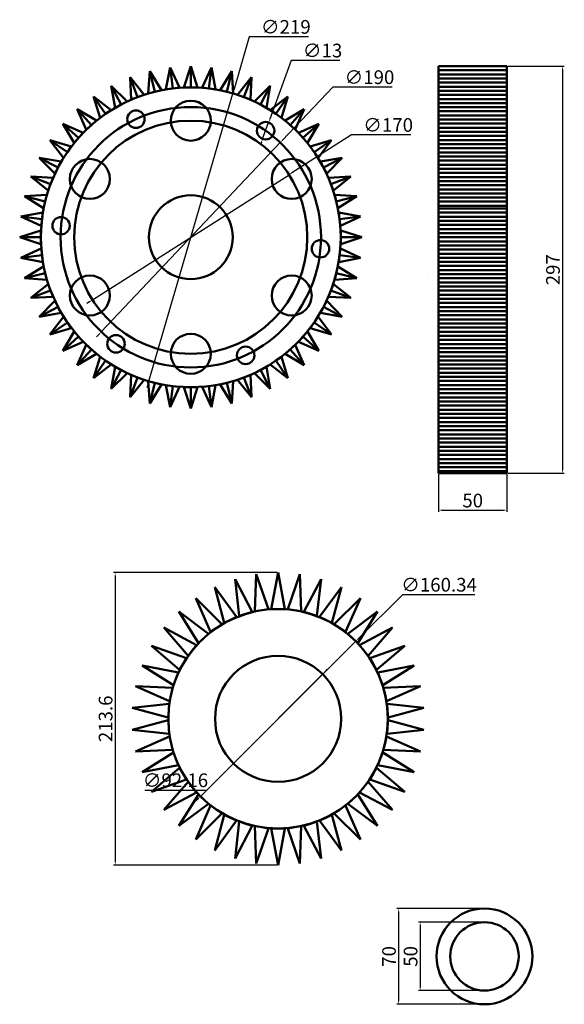
# Model space of a CAD drawing. Units: millimetres. Extents: x 828 to 2987, y 979 to 1807.
# Tile 5 of 6: x 1664 to 2062, y 1028 to 1747. Entities that reach past the tile are written whole.
import ezdxf

# ---------------------------------------------------------------- set-up
doc = ezdxf.new("R2010")
doc.units = ezdxf.units.MM
doc.layers.add('M-DIMS', color=2, linetype='Continuous', lineweight=25)
doc.layers.add('M-OUTL', color=7, linetype='Continuous', lineweight=50)
doc.styles.get("Standard").update_dxf_attribs({"font": 'arial.ttf'})
doc.dimstyles.new('ISO-25', dxfattribs={"dimtxt": 10, "dimasz": 2.5, "dimexe": 1.25, "dimexo": 0.625, "dimtad": 1, "dimtoh": 1, "dimdec": 0, "dimtxsty": 'Standard', "dimcen": 2.5, "dimadec": 0, "dimazin": 0, "dimtfac": 1, "dimtdec": 0, "dimtmove": 0, "dimatfit": 3, "dimfxl": 1, "dimarcsym": 0})

# ---------------------------------------------------------------- blocks, each defined once
blk = doc.blocks.new('*U45')
for p, q in [((-5, -7.75), (0, 7.75)), ((0, -7.75), (0, 7.75)), ((5, -7.75), (0, 7.75)), ((0, -7.75), (-5, -7.75)), ((0, -7.75), (5, -7.75))]:
    blk.add_line(p, q)
blk = doc.blocks.new('*U46')
at = {"layer": 'M-OUTL', "color": 0, "linetype": 'ByBlock', "lineweight": -2, "transparency": 16777216}
for p, rotation in [((1775.03, 1704.64), 6.923076923076879), ((1803.3, 1704.64), 353.0769230769231), ((1747.59, 1697.88), 20.76923076923077), ((1761.1, 1702.09), 13.84615384615382), ((1817.23, 1702.09), 346.1538461538462), ((1830.74, 1697.88), 339.2307692307692), ((1734.67, 1692.07), 27.69230769230768), ((1843.66, 1692.07), 332.3076923076923), ((1722.56, 1684.74), 34.61538461538462), ((1855.77, 1684.74), 325.3846153846154), ((1711.41, 1676.01), 41.53846153846155), ((1866.92, 1676.01), 318.4615384615384), ((1701.4, 1666), 48.46153846153847), ((1876.93, 1666), 311.5384615384616), ((1692.67, 1654.85), 55.38461538461539), ((1885.66, 1654.85), 304.6153846153846), ((1685.34, 1642.74), 62.30769230769233), ((1892.99, 1642.74), 297.6923076923078), ((1679.53, 1629.82), 69.23076923076925), ((1898.8, 1629.82), 290.7692307692308), ((1675.32, 1616.31), 76.15384615384616), ((1903.01, 1616.31), 283.8461538461539), ((1672.77, 1602.38), 83.07692307692308), ((1905.56, 1602.38), 276.923076923077), ((1671.91, 1588.25), 90), ((1906.42, 1588.25), 270.0000000000001), ((1672.77, 1574.11), 96.92307692307695), ((1905.56, 1574.11), 263.0769230769231), ((1675.32, 1560.19), 103.8461538461538), ((1903.01, 1560.19), 256.1538461538462), ((1679.53, 1546.67), 110.7692307692307), ((1898.8, 1546.67), 249.2307692307693), ((1685.34, 1533.76), 117.6923076923077), ((1892.99, 1533.76), 242.3076923076923), ((1692.67, 1521.64), 124.6153846153846), ((1885.66, 1521.64), 235.3846153846154), ((1701.4, 1510.49), 131.5384615384615), ((1876.93, 1510.49), 228.4615384615384), ((1711.41, 1500.48), 138.4615384615385), ((1866.92, 1500.48), 221.5384615384615), ((1722.56, 1491.75), 145.3846153846154), ((1855.77, 1491.75), 214.6153846153847), ((1734.67, 1484.42), 152.3076923076923), ((1843.66, 1484.42), 207.6923076923077), ((1747.59, 1478.61), 159.2307692307692), ((1761.1, 1474.4), 166.1538461538462), ((1817.23, 1474.4), 193.8461538461538), ((1830.74, 1478.61), 200.7692307692307), ((1775.03, 1471.85), 173.0769230769231), ((1789.16, 1470.99), 180), ((1803.3, 1471.85), 186.9230769230768)]:
    blk.add_blockref('*U45', p, dxfattribs=dict(at, rotation=rotation))
blk.add_blockref('*U45', (1789.16, 1705.5), dxfattribs=at)
blk = doc.blocks.new('*U47')
blk.add_circle((0, 0), 14.61)
blk = doc.blocks.new('*U48')
at = {"layer": 'M-OUTL', "color": 0, "linetype": 'ByBlock', "lineweight": -2, "transparency": 16777216}
blk.add_blockref('*U47', (1789.16, 1673.38), dxfattribs=at)
for p, rotation in [((1715.43, 1630.81), 59.99999999999999), ((1862.9, 1630.81), 300), ((1715.43, 1545.68), 120), ((1862.9, 1545.68), 240), ((1789.16, 1503.11), 180)]:
    blk.add_blockref('*U47', p, dxfattribs=dict(at, rotation=rotation))
blk = doc.blocks.new('*U49')
blk.add_circle((0, 0), 6.37)
blk = doc.blocks.new('*U50')
at = {"layer": 'M-OUTL', "color": 0, "linetype": 'ByBlock', "lineweight": -2, "transparency": 16777216}
blk.add_blockref('*U49', (1749.08, 1674.51), dxfattribs=at)
for p, rotation in [((1843.83, 1666.09), 300), ((1694.41, 1596.66), 60), ((1883.92, 1579.83), 239.9999999999999), ((1734.5, 1510.4), 120), ((1829.25, 1501.98), 180)]:
    blk.add_blockref('*U49', p, dxfattribs=dict(at, rotation=rotation))
blk = doc.blocks.new('*D51')
at = {"layer": 'Defpoints', "color": 0, "transparency": 16777216}
for p in [(1970.13, 1415.79), (2020.13, 1415.79), (2020.13, 1388.87)]:
    blk.add_point(p, dxfattribs=at)
at = {"layer": 'M-DIMS', "color": 0, "lineweight": -2, "transparency": 16777216}
for p, q in [((1970.13, 1415.16), (1970.13, 1387.62)), ((2020.13, 1415.16), (2020.13, 1387.62)), ((1972.63, 1388.87), (2017.63, 1388.87))]:
    blk.add_line(p, q, dxfattribs=at)
at = {"layer": 'M-DIMS', "color": 0, "transparency": 16777216}
for points in [[(1972.63, 1389.29), (1972.63, 1388.45), (1970.13, 1388.87)], [(2017.63, 1389.29), (2017.63, 1388.45), (2020.13, 1388.87)]]:
    blk.add_solid(points, dxfattribs=at)
at = {"layer": 'M-DIMS', "color": 0, "transparency": 16777216, "insert": (1995.13, 1394.6), "char_height": 10, "attachment_point": 5}
blk.add_mtext('50', dxfattribs=at)
blk = doc.blocks.new('*D52')
at = {"layer": 'Defpoints', "color": 0, "transparency": 16777216}
for p in [(2020.13, 1713.25), (2020.13, 1415.79), (2060.79, 1415.79)]:
    blk.add_point(p, dxfattribs=at)
at = {"layer": 'M-DIMS', "color": 0, "lineweight": -2, "transparency": 16777216}
for p, q in [((2020.76, 1713.25), (2062.04, 1713.25)), ((2060.79, 1710.75), (2060.79, 1418.29)), ((2020.76, 1415.79), (2062.04, 1415.79))]:
    blk.add_line(p, q, dxfattribs=at)
at = {"layer": 'M-DIMS', "color": 0, "transparency": 16777216}
for points in [[(2060.38, 1710.75), (2061.21, 1710.75), (2060.79, 1713.25)], [(2060.38, 1418.29), (2061.21, 1418.29), (2060.79, 1415.79)]]:
    blk.add_solid(points, dxfattribs=at)
at = {"layer": 'M-DIMS', "color": 0, "transparency": 16777216, "insert": (2055.06, 1564.52), "char_height": 10, "attachment_point": 5, "rotation": 90}
blk.add_mtext('297', dxfattribs=at)
blk = doc.blocks.new('*D53')
at = {"layer": 'Defpoints', "color": 0, "transparency": 16777216}
for p in [(1819.8, 1693.38), (1758.53, 1483.11)]:
    blk.add_point(p, dxfattribs=at)
at = {"layer": 'M-DIMS', "color": 0, "lineweight": -2, "transparency": 16777216}
for p, q in [((1831.82, 1734.62), (1820.5, 1695.78)), ((1875.09, 1734.62), (1831.82, 1734.62)), ((1758.53, 1483.11), (1819.8, 1693.38)), ((1757.83, 1480.71), (1757.13, 1478.31))]:
    blk.add_line(p, q, dxfattribs=at)
at = {"layer": 'M-DIMS', "color": 0, "transparency": 16777216}
for points in [[(1820.1, 1695.9), (1820.9, 1695.66), (1819.8, 1693.38)], [(1757.43, 1480.83), (1758.23, 1480.59), (1758.53, 1483.11)]]:
    blk.add_solid(points, dxfattribs=at)
at = {"layer": 'M-DIMS', "color": 0, "transparency": 16777216, "insert": (1858.59, 1740.63), "char_height": 10, "attachment_point": 5}
blk.add_mtext('∅219', dxfattribs=at)
blk = doc.blocks.new('*D54')
at = {"layer": 'Defpoints', "color": 0, "transparency": 16777216}
for p in [(1854.53, 1657.36), (1723.8, 1519.13)]:
    blk.add_point(p, dxfattribs=at)
at = {"layer": 'M-DIMS', "color": 0, "lineweight": -2, "transparency": 16777216}
for p, q in [((1892.84, 1697.87), (1856.24, 1659.18)), ((1936.17, 1697.87), (1892.84, 1697.87)), ((1723.8, 1519.13), (1854.53, 1657.36)), ((1722.09, 1517.31), (1720.37, 1515.5))]:
    blk.add_line(p, q, dxfattribs=at)
at = {"layer": 'M-DIMS', "color": 0, "transparency": 16777216}
for points in [[(1855.94, 1659.46), (1856.55, 1658.89), (1854.53, 1657.36)], [(1721.78, 1517.6), (1722.39, 1517.03), (1723.8, 1519.13)]]:
    blk.add_solid(points, dxfattribs=at)
at = {"layer": 'M-DIMS', "color": 0, "transparency": 16777216, "insert": (1919.7, 1703.88), "char_height": 10, "attachment_point": 5}
blk.add_mtext('∅190', dxfattribs=at)
blk = doc.blocks.new('*D55')
at = {"layer": 'Defpoints', "color": 0, "transparency": 16777216}
for p in [(1846.01, 1672.08), (1841.65, 1660.1)]:
    blk.add_point(p, dxfattribs=at)
at = {"layer": 'M-DIMS', "color": 0, "lineweight": -2, "transparency": 16777216}
for p, q in [((1862.47, 1717.36), (1846.86, 1674.43)), ((1898.05, 1717.36), (1862.47, 1717.36)), ((1841.65, 1660.1), (1846.01, 1672.08)), ((1840.8, 1657.76), (1839.95, 1655.41))]:
    blk.add_line(p, q, dxfattribs=at)
at = {"layer": 'M-DIMS', "color": 0, "transparency": 16777216}
for points in [[(1846.47, 1674.58), (1847.26, 1674.29), (1846.01, 1672.08)], [(1840.41, 1657.9), (1841.19, 1657.61), (1841.65, 1660.1)]]:
    blk.add_solid(points, dxfattribs=at)
at = {"layer": 'M-DIMS', "color": 0, "transparency": 16777216, "insert": (1885.44, 1723.37), "char_height": 10, "attachment_point": 5}
blk.add_mtext('∅13', dxfattribs=at)
blk = doc.blocks.new('*D56')
at = {"layer": 'Defpoints', "color": 0, "transparency": 16777216}
for p in [(1860.98, 1633.97), (1717.35, 1542.52)]:
    blk.add_point(p, dxfattribs=at)
at = {"layer": 'M-DIMS', "color": 0, "lineweight": -2, "transparency": 16777216}
for p, q in [((1906.52, 1662.97), (1863.09, 1635.32)), ((1949.82, 1662.97), (1906.52, 1662.97)), ((1717.35, 1542.52), (1860.98, 1633.97)), ((1715.24, 1541.18), (1713.13, 1539.83))]:
    blk.add_line(p, q, dxfattribs=at)
at = {"layer": 'M-DIMS', "color": 0, "transparency": 16777216}
for points in [[(1862.86, 1635.67), (1863.31, 1634.96), (1860.98, 1633.97)], [(1715.02, 1541.53), (1715.47, 1540.82), (1717.35, 1542.52)]]:
    blk.add_solid(points, dxfattribs=at)
at = {"layer": 'M-DIMS', "color": 0, "transparency": 16777216, "insert": (1933.35, 1668.98), "char_height": 10, "attachment_point": 5}
blk.add_mtext('∅170', dxfattribs=at)
blk = doc.blocks.new('*U57')
for p, q in [((-5, -13.32), (0, 13.32)), ((5, -13.32), (0, 13.32)), ((0, -13.32), (-5, -13.32)), ((0, -13.32), (5, -13.32))]:
    blk.add_line(p, q)
blk = doc.blocks.new('*U58')
at = {"layer": 'M-OUTL', "color": 0, "linetype": 'ByBlock', "lineweight": -2, "transparency": 16777216}
for p, rotation in [((1825.4, 1325.77), 17.14285714285713), ((1839.02, 1328.88), 8.571428571428495), ((1866.89, 1328.88), 351.4285714285715), ((1880.51, 1325.77), 342.8571428571429), ((1812.39, 1320.67), 25.71428571428572), ((1893.52, 1320.67), 334.2857142857143), ((1800.29, 1313.68), 34.28571428571429), ((1905.62, 1313.68), 325.7142857142857), ((1789.37, 1304.97), 42.85714285714287), ((1916.54, 1304.97), 317.1428571428572), ((1779.86, 1294.72), 51.42857142857143), ((1926.05, 1294.72), 308.5714285714286), ((1771.99, 1283.18), 60), ((1933.92, 1283.18), 300), ((1765.93, 1270.59), 68.57142857142858), ((1939.98, 1270.59), 291.4285714285714), ((1761.81, 1257.24), 77.14285714285714), ((1944.1, 1257.24), 282.8571428571428), ((1759.73, 1243.42), 85.71428571428572), ((1946.18, 1243.42), 274.2857142857143), ((1759.73, 1229.45), 94.28571428571432), ((1946.18, 1229.45), 265.7142857142857), ((1761.81, 1215.63), 102.8571428571428), ((1944.1, 1215.63), 257.1428571428572), ((1765.93, 1202.28), 111.4285714285714), ((1939.98, 1202.28), 248.5714285714286), ((1771.99, 1189.69), 120), ((1933.92, 1189.69), 240), ((1779.86, 1178.15), 128.5714285714286), ((1926.05, 1178.15), 231.4285714285714), ((1789.37, 1167.9), 137.1428571428571), ((1916.54, 1167.9), 222.8571428571428), ((1800.29, 1159.19), 145.7142857142857), ((1905.62, 1159.19), 214.2857142857143), ((1812.39, 1152.21), 154.2857142857143), ((1893.52, 1152.21), 205.7142857142857), ((1825.4, 1147.1), 162.8571428571429), ((1880.51, 1147.1), 197.1428571428571), ((1839.02, 1143.99), 171.4285714285715), ((1852.96, 1142.95), 180), ((1866.89, 1143.99), 188.5714285714286)]:
    blk.add_blockref('*U57', p, dxfattribs=dict(at, rotation=rotation))
blk.add_blockref('*U57', (1852.96, 1329.92), dxfattribs=at)
blk = doc.blocks.new('*D59')
at = {"layer": 'Defpoints', "color": 0, "transparency": 16777216}
for p in [(2003.72, 1097.86), (1941, 1027.86), (2003.72, 1027.86)]:
    blk.add_point(p, dxfattribs=at)
at = {"layer": 'M-DIMS', "color": 0, "lineweight": -2, "transparency": 16777216}
for p, q in [((2003.09, 1097.86), (1939.75, 1097.86)), ((1941, 1095.36), (1941, 1030.36)), ((2003.09, 1027.86), (1939.75, 1027.86))]:
    blk.add_line(p, q, dxfattribs=at)
at = {"layer": 'M-DIMS', "color": 0, "transparency": 16777216}
for points in [[(1940.58, 1095.36), (1941.42, 1095.36), (1941, 1097.86)], [(1940.58, 1030.36), (1941.42, 1030.36), (1941, 1027.86)]]:
    blk.add_solid(points, dxfattribs=at)
at = {"layer": 'M-DIMS', "color": 0, "transparency": 16777216, "insert": (1935.27, 1062.86), "char_height": 10, "attachment_point": 5, "rotation": 90}
blk.add_mtext('70', dxfattribs=at)
blk = doc.blocks.new('*D60')
at = {"layer": 'Defpoints', "color": 0, "transparency": 16777216}
for p in [(2003.72, 1087.86), (1956.76, 1037.86), (2003.72, 1037.86)]:
    blk.add_point(p, dxfattribs=at)
at = {"layer": 'M-DIMS', "color": 0, "lineweight": -2, "transparency": 16777216}
for p, q in [((2003.09, 1087.86), (1955.51, 1087.86)), ((1956.76, 1085.36), (1956.76, 1040.36)), ((2003.09, 1037.86), (1955.51, 1037.86))]:
    blk.add_line(p, q, dxfattribs=at)
at = {"layer": 'M-DIMS', "color": 0, "transparency": 16777216}
for points in [[(1956.34, 1085.36), (1957.18, 1085.36), (1956.76, 1087.86)], [(1956.34, 1040.36), (1957.18, 1040.36), (1956.76, 1037.86)]]:
    blk.add_solid(points, dxfattribs=at)
at = {"layer": 'M-DIMS', "color": 0, "transparency": 16777216, "insert": (1951.03, 1062.86), "char_height": 10, "attachment_point": 5, "rotation": 90}
blk.add_mtext('50', dxfattribs=at)
blk = doc.blocks.new('*D98')
at = {"layer": 'Defpoints', "color": 0, "transparency": 16777216}
for p in [(1852.96, 1343.24), (1733.95, 1129.63), (1852.96, 1129.63)]:
    blk.add_point(p, dxfattribs=at)
at = {"layer": 'M-DIMS', "color": 0, "lineweight": -2, "transparency": 16777216}
for p, q in [((1852.33, 1343.24), (1732.7, 1343.24)), ((1733.95, 1340.74), (1733.95, 1132.13)), ((1852.33, 1129.63), (1732.7, 1129.63))]:
    blk.add_line(p, q, dxfattribs=at)
at = {"layer": 'M-DIMS', "color": 0, "transparency": 16777216}
for points in [[(1733.54, 1340.74), (1734.37, 1340.74), (1733.95, 1343.24)], [(1733.54, 1132.13), (1734.37, 1132.13), (1733.95, 1129.63)]]:
    blk.add_solid(points, dxfattribs=at)
at = {"layer": 'M-DIMS', "color": 0, "transparency": 16777216, "insert": (1728.22, 1236.44), "char_height": 10, "attachment_point": 5, "rotation": 90}
blk.add_mtext('213.6', dxfattribs=at)
blk = doc.blocks.new('*D139')
at = {"layer": 'Defpoints', "color": 0, "transparency": 16777216}
for p in [(1909.69, 1293.09), (1796.23, 1179.78)]:
    blk.add_point(p, dxfattribs=at)
at = {"layer": 'M-DIMS', "color": 0, "lineweight": -2, "transparency": 16777216}
for p, q in [((1943.72, 1327.08), (1911.46, 1294.85)), ((1996.7, 1327.08), (1943.72, 1327.08)), ((1796.23, 1179.78), (1909.69, 1293.09)), ((1794.46, 1178.02), (1792.69, 1176.25))]:
    blk.add_line(p, q, dxfattribs=at)
at = {"layer": 'M-DIMS', "color": 0, "transparency": 16777216}
for points in [[(1911.16, 1295.15), (1911.75, 1294.56), (1909.69, 1293.09)], [(1794.16, 1178.31), (1794.75, 1177.72), (1796.23, 1179.78)]]:
    blk.add_solid(points, dxfattribs=at)
at = {"layer": 'M-DIMS', "color": 0, "transparency": 16777216, "insert": (1970.53, 1333.09), "char_height": 10, "attachment_point": 5}
blk.add_mtext('∅160.34', dxfattribs=at)
blk = doc.blocks.new('*D140')
at = {"layer": 'Defpoints', "color": 0, "transparency": 16777216}
for p in [(1885.5, 1269.06), (1820.41, 1203.81)]:
    blk.add_point(p, dxfattribs=at)
at = {"layer": 'M-DIMS', "color": 0, "lineweight": -2, "transparency": 16777216}
for p, q in [((1885.5, 1269.06), (1820.41, 1203.81)), ((1887.27, 1270.83), (1889.03, 1272.6)), ((1800.88, 1184.24), (1818.65, 1202.04)), ((1755.64, 1184.24), (1800.88, 1184.24))]:
    blk.add_line(p, q, dxfattribs=at)
at = {"layer": 'M-DIMS', "color": 0, "transparency": 16777216}
for points in [[(1886.97, 1271.12), (1887.56, 1270.54), (1885.5, 1269.06)], [(1818.35, 1202.34), (1818.94, 1201.75), (1820.41, 1203.81)]]:
    blk.add_solid(points, dxfattribs=at)
at = {"layer": 'M-DIMS', "color": 0, "transparency": 16777216, "insert": (1777.95, 1190.25), "char_height": 10, "attachment_point": 5}
blk.add_mtext('∅92.16', dxfattribs=at)

msp = doc.modelspace()

# ---------------------------------------------------------------- linework, layer by layer
at = {"layer": 'M-OUTL'}
for p, q in [((1970.132, 1713.2458), (1970.132, 1415.7856)), ((1970.132, 1713.2458), (2020.132, 1713.2458)), ((1970.132, 1713.2458), (1970.132, 1710.2458)), ((2020.132, 1713.2458), (2020.132, 1415.7856)), ((1970.132, 1710.2458), (2020.132, 1710.2458)), ((2020.132, 1707.2458), (1970.132, 1707.2458)), ((1970.132, 1704.2458), (2020.132, 1704.2458)), ((2020.132, 1701.2458), (1970.132, 1701.2458)), ((1970.132, 1698.2458), (2020.132, 1698.2458)), ((2020.132, 1695.2458), (1970.132, 1695.2458)), ((1970.132, 1692.2458), (2020.132, 1692.2458)), ((1747.9972, 1689.7212), (1747.9951, 1689.7512)), ((2020.132, 1689.2458), (1970.132, 1689.2458)), ((1970.132, 1686.2458), (2020.132, 1686.2458)), ((2020.132, 1683.2458), (1970.132, 1683.2458)), ((1970.132, 1680.2458), (2020.132, 1680.2458)), ((2020.132, 1677.2458), (1970.132, 1677.2458)), ((1970.132, 1674.2458), (2020.132, 1674.2458)), ((2020.132, 1671.2458), (1970.132, 1671.2458)), ((1970.132, 1668.2458), (2020.132, 1668.2458)), ((2020.132, 1665.2458), (1970.132, 1665.2458)), ((1970.132, 1662.2458), (2020.132, 1662.2458)), ((2020.132, 1659.2458), (1970.132, 1659.2458)), ((1970.132, 1656.2458), (2020.132, 1656.2458)), ((2020.132, 1653.2458), (1970.132, 1653.2458)), ((1970.132, 1650.2458), (2020.132, 1650.2458)), ((2020.132, 1647.2458), (1970.132, 1647.2458)), ((1970.132, 1644.2458), (2020.132, 1644.2458)), ((2020.132, 1641.2458), (1970.132, 1641.2458)), ((1970.132, 1638.2458), (2020.132, 1638.2458)), ((2020.132, 1635.2458), (1970.132, 1635.2458)), ((1970.132, 1632.2458), (2020.132, 1632.2458)), ((2020.132, 1629.2458), (1970.132, 1629.2458)), ((1970.132, 1626.2458), (2020.132, 1626.2458)), ((2020.132, 1623.2458), (1970.132, 1623.2458)), ((1970.132, 1620.2458), (2020.132, 1620.2458)), ((2020.132, 1617.2458), (1970.132, 1617.2458)), ((1970.132, 1614.2458), (2020.132, 1614.2458)), ((2020.132, 1611.2458), (1970.132, 1611.2458)), ((1970.132, 1609.2458), (2020.132, 1609.2458)), ((2020.132, 1606.2458), (1970.132, 1606.2458)), ((1970.132, 1603.2458), (2020.132, 1603.2458)), ((2020.132, 1600.2458), (1970.132, 1600.2458)), ((1970.132, 1597.2458), (2020.132, 1597.2458)), ((2020.132, 1594.2458), (1970.132, 1594.2458)), ((1970.132, 1591.2458), (2020.132, 1591.2458)), ((2020.132, 1588.2458), (1970.132, 1588.2458)), ((1970.132, 1585.2458), (2020.132, 1585.2458)), ((2020.132, 1582.2458), (1970.132, 1582.2458)), ((1970.132, 1579.2458), (2020.132, 1579.2458)), ((2020.132, 1576.2458), (1970.132, 1576.2458)), ((1970.132, 1573.2458), (2020.132, 1573.2458)), ((2020.132, 1570.2458), (1970.132, 1570.2458)), ((1970.132, 1567.2458), (2020.132, 1567.2458)), ((2020.132, 1564.2458), (1970.132, 1564.2458)), ((1970.132, 1561.2458), (2020.132, 1561.2458)), ((1962.5354, 1558.2458), (1962.5354, 1558.2458)), ((2020.132, 1558.2458), (1970.132, 1558.2458)), ((1970.132, 1555.2458), (2020.132, 1555.2458)), ((2020.132, 1552.2458), (1970.132, 1552.2458)), ((1970.132, 1549.2458), (2020.132, 1549.2458)), ((2020.132, 1546.2458), (1970.132, 1546.2458)), ((1970.132, 1543.2458), (2020.132, 1543.2458)), ((2020.132, 1540.2458), (1970.132, 1540.2458)), ((1970.132, 1537.2458), (2020.132, 1537.2458)), ((2020.132, 1534.2458), (1970.132, 1534.2458)), ((1970.132, 1531.2458), (2020.132, 1531.2458)), ((2020.132, 1528.2458), (1970.132, 1528.2458)), ((1970.132, 1525.2458), (2020.132, 1525.2458)), ((2020.132, 1522.2458), (1970.132, 1522.2458)), ((1970.132, 1519.2458), (2020.132, 1519.2458)), ((2020.132, 1516.2458), (1970.132, 1516.2458)), ((1970.132, 1513.2458), (2020.132, 1513.2458)), ((2020.132, 1510.2458), (1970.132, 1510.2458)), ((1970.132, 1507.2458), (2020.132, 1507.2458)), ((2020.132, 1504.2458), (1970.132, 1504.2458)), ((1970.132, 1501.2458), (2020.132, 1501.2458)), ((2020.132, 1498.2458), (1970.132, 1498.2458)), ((1970.132, 1495.2458), (2020.132, 1495.2458)), ((2020.132, 1492.2458), (1970.132, 1492.2458)), ((1970.132, 1489.2458), (2020.132, 1489.2458)), ((2020.132, 1486.2458), (1970.132, 1486.2458)), ((1970.132, 1483.2458), (2020.132, 1483.2458)), ((2020.132, 1480.2458), (1970.132, 1480.2458)), ((1970.132, 1477.2458), (2020.132, 1477.2458)), ((2020.132, 1474.2458), (1970.132, 1474.2458)), ((1970.132, 1471.2458), (2020.132, 1471.2458)), ((2020.132, 1468.2458), (1970.132, 1468.2458)), ((1970.132, 1465.2458), (2020.132, 1465.2458)), ((2020.132, 1462.2458), (1970.132, 1462.2458)), ((1970.132, 1459.2458), (2020.132, 1459.2458)), ((2020.132, 1456.2458), (1970.132, 1456.2458)), ((1970.132, 1453.2458), (2020.132, 1453.2458)), ((2020.132, 1450.2458), (1970.132, 1450.2458)), ((1970.132, 1447.2458), (2020.132, 1447.2458)), ((2020.132, 1444.2458), (1970.132, 1444.2458)), ((1970.132, 1441.2458), (2020.132, 1441.2458)), ((2020.132, 1438.2458), (1970.132, 1438.2458)), ((1970.132, 1435.2458), (2020.132, 1435.2458)), ((2020.132, 1432.2458), (1970.132, 1432.2458)), ((1970.132, 1429.2458), (2020.132, 1429.2458)), ((2020.132, 1426.2458), (1970.132, 1426.2458)), ((1970.132, 1423.2458), (2020.132, 1423.2458)), ((2020.132, 1420.2458), (1970.132, 1420.2458)), ((1970.132, 1417.2458), (2020.132, 1417.2458)), ((1970.132, 1415.7856), (2020.132, 1415.7856))]:
    msp.add_line(p, q, dxfattribs=at)
for centre, radius in [((1789.1648, 1588.2458), 109.5081), ((1789.1648, 1588.2458), 95.1258), ((1789.1648, 1588.2458), 85.1372), ((1789.1648, 1588.2458), 30.6303), ((1852.9562, 1236.4356), 80.1723), ((1852.9562, 1236.4356), 46.0813), ((2003.7164, 1062.8615), 35), ((2003.7164, 1062.8615), 25)]:
    msp.add_circle(centre, radius, dxfattribs=at)

# ---------------------------------------------------------------- block references
for name in ['*U46', '*U48', '*U50', '*U58']:
    msp.add_blockref(name, (0, 0), dxfattribs=at)

# ---------------------------------------------------------------- dimensions: what is measured, and where the dimension line sits
at = {"layer": 'M-DIMS'}
for p1, p2, override, picture, middle in [((1758.5261, 1483.1111), (1819.8034, 1693.3805), {"dimclrd": 0, "dimclre": 0, "dimclrt": 0}, '*D53', (1858.5918, 1734.6175)), ((1841.6548, 1660.1047), (1846.0096, 1672.0838), {"dimclrd": 0, "dimclre": 0, "dimclrt": 0}, '*D55', (1885.4432, 1717.3585)), ((1723.8039, 1519.1309), (1854.5256, 1657.3607), {"dimclrd": 0, "dimclre": 0, "dimclrt": 0}, '*D54', (1919.6968, 1697.8726)), ((1717.3504, 1542.5179), (1860.9792, 1633.9737), {"dimclrd": 0, "dimclre": 0, "dimclrt": 0}, '*D56', (1933.3465, 1662.9746)), ((1796.2261, 1179.7848), (1909.6862, 1293.0863), {"dimdec": 2, "dimlfac": 1, "dimrnd": 0, "dimzin": 0, "dimdsep": 46, "dimlunit": 2}, '*D139', (1970.5259, 1327.0767)), ((1885.5009, 1269.0596), (1820.4114, 1203.8115), {"dimdec": 2, "dimlfac": 1, "dimrnd": 0, "dimzin": 0, "dimdsep": 46, "dimlunit": 2}, '*D140', (1777.9506, 1184.237))]:
    dim = msp.add_diameter_dim_2p(p1=p1, p2=p2, dimstyle='ISO-25', override=override, dxfattribs=at)
    dim.commit()
    dim.dimension.update_dxf_attribs({"geometry": picture, "text_midpoint": middle, "dimtype": 163})
for base, p1, p2, override, picture, middle in [((2060.7926, 1415.7856), (2020.132, 1713.2458), (2020.132, 1415.7856), {"dimclrd": 0, "dimclre": 0, "dimclrt": 0}, '*D52', (2055.0619, 1564.5157)), ((1733.9517, 1129.6325), (1852.9562, 1343.2386), (1852.9562, 1129.6325), {"dimdec": 1, "dimlfac": 1, "dimrnd": 0, "dimzin": 0, "dimdsep": 46, "dimlunit": 2}, '*D98', (1728.2176, 1236.4355)), ((1941.0006, 1027.8615), (2003.7164, 1097.8615), (2003.7164, 1027.8615), {"dimclrd": 0, "dimclre": 0, "dimclrt": 0}, '*D59', (1935.2699, 1062.8615)), ((1956.7596, 1037.8615), (2003.7164, 1087.8615), (2003.7164, 1037.8615), {"dimclrd": 0, "dimclre": 0, "dimclrt": 0}, '*D60', (1951.0289, 1062.8615))]:
    dim = msp.add_linear_dim(base=base, p1=p1, p2=p2, angle=90, dimstyle='ISO-25', override=override, dxfattribs=at)
    dim.commit()
    dim.dimension.update_dxf_attribs({"geometry": picture, "text_midpoint": middle})
dim = msp.add_linear_dim(base=(2020.132, 1388.8711), p1=(1970.132, 1415.7856), p2=(2020.132, 1415.7856), dimstyle='ISO-25', override={"dimclrd": 0, "dimclre": 0, "dimclrt": 0}, dxfattribs=at)
dim.commit()
dim.dimension.update_dxf_attribs({"geometry": '*D51', "text_midpoint": (1995.132, 1394.6018)})

doc.saveas('drawing.dxf')
